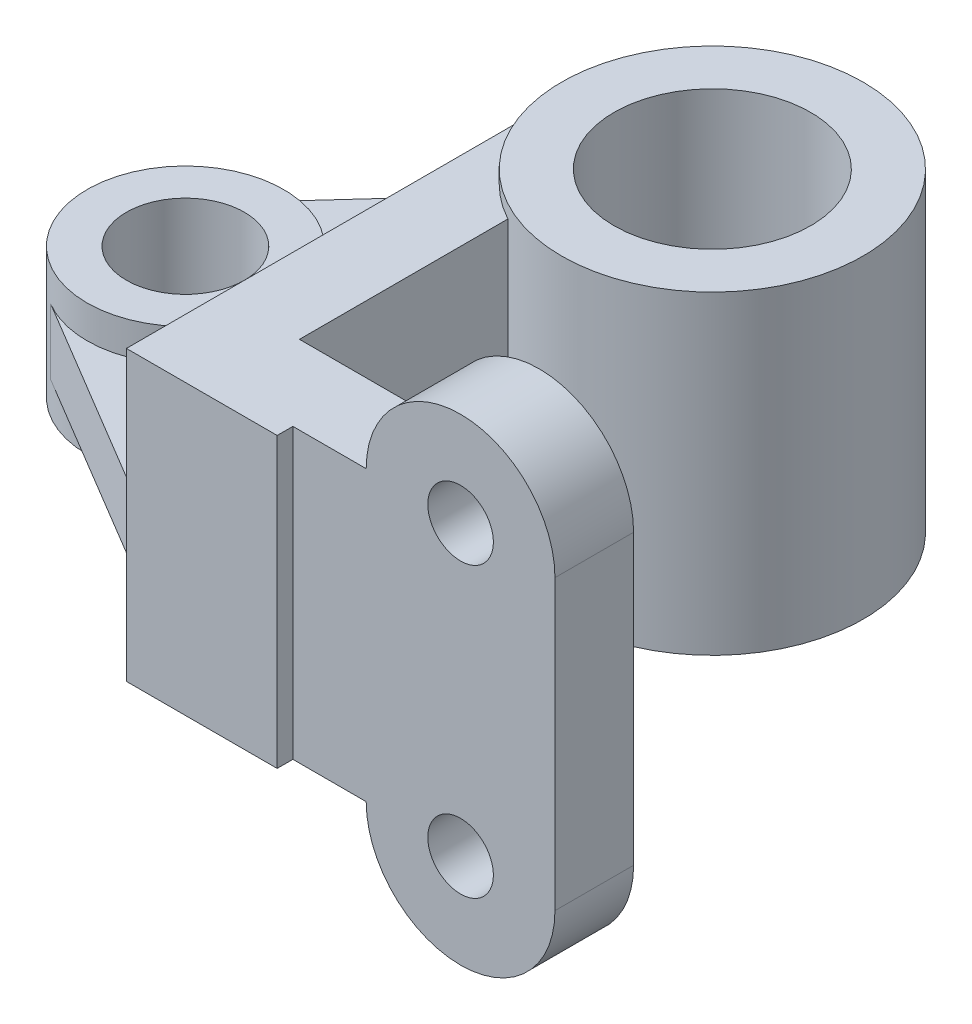
ISO-10303-21;
HEADER;
FILE_DESCRIPTION(('STEP AP214'),'2;1');
FILE_NAME('part.step','',(''),(''),'','','');
FILE_SCHEMA(('AUTOMOTIVE_DESIGN { 1 0 10303 214 1 1 1 1 }'));
ENDSEC;
DATA;
#1=APPLICATION_CONTEXT('core data for automotive mechanical design processes');
#2=APPLICATION_PROTOCOL_DEFINITION('international standard','automotive_design',2000,#1);
#3=PRODUCT_CONTEXT('',#1,'mechanical');
#4=PRODUCT('Part','Part','',(#3));
#5=PRODUCT_RELATED_PRODUCT_CATEGORY('part','',(#4));
#6=PRODUCT_DEFINITION_FORMATION('','',#4);
#7=PRODUCT_DEFINITION_CONTEXT('part definition',#1,'design');
#8=PRODUCT_DEFINITION('design','',#6,#7);
#9=PRODUCT_DEFINITION_SHAPE('','',#8);
#10=(LENGTH_UNIT() NAMED_UNIT(*) SI_UNIT(.MILLI.,.METRE.));
#11=(NAMED_UNIT(*) PLANE_ANGLE_UNIT() SI_UNIT($,.RADIAN.));
#12=(NAMED_UNIT(*) SI_UNIT($,.STERADIAN.) SOLID_ANGLE_UNIT());
#13=UNCERTAINTY_MEASURE_WITH_UNIT(LENGTH_MEASURE(1.E-05),#10,'distance_accuracy_value','');
#14=(GEOMETRIC_REPRESENTATION_CONTEXT(3) GLOBAL_UNCERTAINTY_ASSIGNED_CONTEXT((#13)) GLOBAL_UNIT_ASSIGNED_CONTEXT((#10,
#11,#12)) REPRESENTATION_CONTEXT('',''));
#15=CARTESIAN_POINT('',(0.,0.,0.));
#16=DIRECTION('',(0.,0.,1.));
#17=DIRECTION('',(1.,0.,0.));
#18=AXIS2_PLACEMENT_3D('',#15,#16,#17);
#19=CARTESIAN_POINT('',(55.2083333333334,-55.,0.));
#20=DIRECTION('',(0.,0.,1.));
#21=DIRECTION('',(1.,0.,0.));
#22=AXIS2_PLACEMENT_3D('',#19,#20,#21);
#23=PLANE('',#22);
#24=CARTESIAN_POINT('',(55.2083333333334,55.,0.));
#25=DIRECTION('',(0.,0.,1.));
#26=DIRECTION('',(1.,0.,0.));
#27=AXIS2_PLACEMENT_3D('',#24,#25,#26);
#28=CIRCLE('',#27,30.);
#29=CARTESIAN_POINT('',(85.2083333333334,55.,0.));
#30=VERTEX_POINT('',#29);
#31=EDGE_CURVE('E47',#30,#30,#28,.F.);
#32=ORIENTED_EDGE('',*,*,#31,.F.);
#33=EDGE_LOOP('',(#32));
#34=FACE_BOUND('',#33,.T.);
#35=DIRECTION('',(0.,-1.,0.));
#36=VECTOR('',#35,1.);
#37=CARTESIAN_POINT('',(-36.25,55.,0.));
#38=LINE('',#37,#36);
#39=CARTESIAN_POINT('',(-36.25,55.,0.));
#40=VERTEX_POINT('',#39);
#41=CARTESIAN_POINT('',(-36.25,-55.,0.));
#42=VERTEX_POINT('',#41);
#43=EDGE_CURVE('E212',#40,#42,#38,.T.);
#44=ORIENTED_EDGE('',*,*,#43,.F.);
#45=DIRECTION('',(-1.,0.,0.));
#46=VECTOR('',#45,1.);
#47=CARTESIAN_POINT('',(-66.25,55.,0.));
#48=LINE('',#47,#46);
#49=CARTESIAN_POINT('',(19.2083333333334,54.9999999999999,0.));
#50=VERTEX_POINT('',#49);
#51=EDGE_CURVE('E266',#50,#40,#48,.T.);
#52=ORIENTED_EDGE('',*,*,#51,.F.);
#53=CARTESIAN_POINT('',(55.2083333333334,55.,0.));
#54=DIRECTION('',(0.,0.,1.));
#55=DIRECTION('',(1.,0.,0.));
#56=AXIS2_PLACEMENT_3D('',#53,#54,#55);
#57=CIRCLE('',#56,36.);
#58=CARTESIAN_POINT('',(91.2083333333334,55.,0.));
#59=VERTEX_POINT('',#58);
#60=EDGE_CURVE('E263',#59,#50,#57,.T.);
#61=ORIENTED_EDGE('',*,*,#60,.F.);
#62=DIRECTION('',(0.,1.,0.));
#63=VECTOR('',#62,1.);
#64=CARTESIAN_POINT('',(91.2083333333334,55.,0.));
#65=LINE('',#64,#63);
#66=CARTESIAN_POINT('',(91.2083333333334,-55.0000000000001,0.));
#67=VERTEX_POINT('',#66);
#68=EDGE_CURVE('E257',#67,#59,#65,.T.);
#69=ORIENTED_EDGE('',*,*,#68,.F.);
#70=CARTESIAN_POINT('',(55.2083333333334,-55.,0.));
#71=DIRECTION('',(0.,0.,1.));
#72=DIRECTION('',(1.,0.,0.));
#73=AXIS2_PLACEMENT_3D('',#70,#71,#72);
#74=CIRCLE('',#73,36.);
#75=CARTESIAN_POINT('',(19.2083333333334,-55.,0.));
#76=VERTEX_POINT('',#75);
#77=EDGE_CURVE('E260',#76,#67,#74,.T.);
#78=ORIENTED_EDGE('',*,*,#77,.F.);
#79=DIRECTION('',(1.,0.,0.));
#80=VECTOR('',#79,1.);
#81=CARTESIAN_POINT('',(-66.2499999999999,-55.,0.));
#82=LINE('',#81,#80);
#83=EDGE_CURVE('E250',#42,#76,#82,.T.);
#84=ORIENTED_EDGE('',*,*,#83,.F.);
#85=EDGE_LOOP('',(#44,#52,#61,#69,#78,#84));
#86=FACE_BOUND('',#85,.T.);
#87=CARTESIAN_POINT('',(55.2083333333334,-55.,0.));
#88=DIRECTION('',(0.,0.,1.));
#89=DIRECTION('',(1.,0.,0.));
#90=AXIS2_PLACEMENT_3D('',#87,#88,#89);
#91=CIRCLE('',#90,30.);
#92=CARTESIAN_POINT('',(85.2083333333334,-55.,0.));
#93=VERTEX_POINT('',#92);
#94=EDGE_CURVE('E11',#93,#93,#91,.F.);
#95=ORIENTED_EDGE('',*,*,#94,.F.);
#96=EDGE_LOOP('',(#95));
#97=FACE_BOUND('',#96,.T.);
#98=ADVANCED_FACE('F41',(#34,#86,#97),#23,.F.);
#99=CARTESIAN_POINT('',(-66.25,55.,36.));
#100=DIRECTION('',(1.,0.,0.));
#101=DIRECTION('',(0.,1.,0.));
#102=AXIS2_PLACEMENT_3D('',#99,#100,#101);
#103=PLANE('',#102);
#104=DIRECTION('',(0.,0.,-1.));
#105=VECTOR('',#104,1.);
#106=CARTESIAN_POINT('',(-66.25,-12.5,36.));
#107=LINE('',#106,#105);
#108=CARTESIAN_POINT('',(-66.25,-12.5,36.));
#109=VERTEX_POINT('',#108);
#110=CARTESIAN_POINT('',(-66.25,-12.5,-130.));
#111=VERTEX_POINT('',#110);
#112=EDGE_CURVE('E159',#109,#111,#107,.T.);
#113=ORIENTED_EDGE('',*,*,#112,.T.);
#114=DIRECTION('',(0.,-1.,0.));
#115=VECTOR('',#114,1.);
#116=CARTESIAN_POINT('',(-66.25,55.,-130.));
#117=LINE('',#116,#115);
#118=CARTESIAN_POINT('',(-66.25,-55.,-130.));
#119=VERTEX_POINT('',#118);
#120=EDGE_CURVE('E220',#111,#119,#117,.T.);
#121=ORIENTED_EDGE('',*,*,#120,.T.);
#122=DIRECTION('',(0.,0.,-1.));
#123=VECTOR('',#122,1.);
#124=CARTESIAN_POINT('',(-66.2499999999999,-55.,36.));
#125=LINE('',#124,#123);
#126=CARTESIAN_POINT('',(-66.2499999999999,-55.,36.));
#127=VERTEX_POINT('',#126);
#128=EDGE_CURVE('E276',#127,#119,#125,.T.);
#129=ORIENTED_EDGE('',*,*,#128,.F.);
#130=DIRECTION('',(0.,-1.,0.));
#131=VECTOR('',#130,1.);
#132=CARTESIAN_POINT('',(-66.25,55.,36.));
#133=LINE('',#132,#131);
#134=EDGE_CURVE('E57',#109,#127,#133,.T.);
#135=ORIENTED_EDGE('',*,*,#134,.F.);
#136=EDGE_LOOP('',(#113,#121,#129,#135));
#137=FACE_BOUND('',#136,.T.);
#138=ADVANCED_FACE('F291',(#137),#103,.F.);
#139=CARTESIAN_POINT('',(55.2083333333334,-55.,36.));
#140=DIRECTION('',(0.,0.,1.));
#141=DIRECTION('',(1.,0.,0.));
#142=AXIS2_PLACEMENT_3D('',#139,#140,#141);
#143=PLANE('',#142);
#144=DIRECTION('',(0.,1.,0.));
#145=VECTOR('',#144,1.);
#146=CARTESIAN_POINT('',(-8.74999999999997,-118.,36.));
#147=LINE('',#146,#145);
#148=CARTESIAN_POINT('',(-8.74999999999997,-55.,36.));
#149=VERTEX_POINT('',#148);
#150=CARTESIAN_POINT('',(-8.74999999999997,54.9999999999999,36.));
#151=VERTEX_POINT('',#150);
#152=EDGE_CURVE('E222',#149,#151,#147,.T.);
#153=ORIENTED_EDGE('',*,*,#152,.T.);
#154=DIRECTION('',(-1.,0.,0.));
#155=VECTOR('',#154,1.);
#156=CARTESIAN_POINT('',(-66.25,55.,36.));
#157=LINE('',#156,#155);
#158=CARTESIAN_POINT('',(-66.25,55.,36.));
#159=VERTEX_POINT('',#158);
#160=EDGE_CURVE('E251',#151,#159,#157,.T.);
#161=ORIENTED_EDGE('',*,*,#160,.T.);
#162=CARTESIAN_POINT('',(-66.25,12.5,36.));
#163=VERTEX_POINT('',#162);
#164=EDGE_CURVE('E246',#159,#163,#133,.T.);
#165=ORIENTED_EDGE('',*,*,#164,.T.);
#166=DIRECTION('',(0.,-1.,0.));
#167=VECTOR('',#166,1.);
#168=CARTESIAN_POINT('',(-66.25,12.5,36.));
#169=LINE('',#168,#167);
#170=EDGE_CURVE('E173',#163,#109,#169,.T.);
#171=ORIENTED_EDGE('',*,*,#170,.T.);
#172=ORIENTED_EDGE('',*,*,#134,.T.);
#173=DIRECTION('',(1.,0.,0.));
#174=VECTOR('',#173,1.);
#175=CARTESIAN_POINT('',(-66.2499999999999,-55.,36.));
#176=LINE('',#175,#174);
#177=EDGE_CURVE('E247',#127,#149,#176,.T.);
#178=ORIENTED_EDGE('',*,*,#177,.T.);
#179=EDGE_LOOP('',(#153,#161,#165,#171,#172,#178));
#180=FACE_BOUND('',#179,.T.);
#181=ADVANCED_FACE('F381',(#180),#143,.T.);
#182=CARTESIAN_POINT('',(-66.25,55.,-130.));
#183=VERTEX_POINT('',#182);
#184=CARTESIAN_POINT('',(-66.25,12.5,-130.));
#185=VERTEX_POINT('',#184);
#186=EDGE_CURVE('E217',#183,#185,#117,.T.);
#187=ORIENTED_EDGE('',*,*,#186,.T.);
#188=DIRECTION('',(0.,0.,-1.));
#189=VECTOR('',#188,1.);
#190=CARTESIAN_POINT('',(-66.25,12.5,36.));
#191=LINE('',#190,#189);
#192=EDGE_CURVE('E64',#163,#185,#191,.T.);
#193=ORIENTED_EDGE('',*,*,#192,.F.);
#194=ORIENTED_EDGE('',*,*,#164,.F.);
#195=DIRECTION('',(0.,0.,-1.));
#196=VECTOR('',#195,1.);
#197=CARTESIAN_POINT('',(-66.25,55.,36.));
#198=LINE('',#197,#196);
#199=EDGE_CURVE('E254',#159,#183,#198,.T.);
#200=ORIENTED_EDGE('',*,*,#199,.T.);
#201=EDGE_LOOP('',(#187,#193,#194,#200));
#202=FACE_BOUND('',#201,.T.);
#203=ADVANCED_FACE('F43',(#202),#103,.F.);
#204=CARTESIAN_POINT('',(-66.2499999999999,-55.,36.));
#205=DIRECTION('',(0.,1.,0.));
#206=DIRECTION('',(0.,0.,1.));
#207=AXIS2_PLACEMENT_3D('',#204,#205,#206);
#208=PLANE('',#207);
#209=DIRECTION('',(-1.,0.,0.));
#210=VECTOR('',#209,1.);
#211=CARTESIAN_POINT('',(-66.2499999999999,-55.,30.));
#212=LINE('',#211,#210);
#213=CARTESIAN_POINT('',(19.2083333333334,-55.,30.));
#214=VERTEX_POINT('',#213);
#215=CARTESIAN_POINT('',(-8.74999999999997,-55.,30.));
#216=VERTEX_POINT('',#215);
#217=EDGE_CURVE('E242',#214,#216,#212,.T.);
#218=ORIENTED_EDGE('',*,*,#217,.T.);
#219=DIRECTION('',(0.,0.,1.));
#220=VECTOR('',#219,1.);
#221=CARTESIAN_POINT('',(-8.74999999999997,-55.,36.));
#222=LINE('',#221,#220);
#223=EDGE_CURVE('E244',#216,#149,#222,.T.);
#224=ORIENTED_EDGE('',*,*,#223,.T.);
#225=ORIENTED_EDGE('',*,*,#177,.F.);
#226=ORIENTED_EDGE('',*,*,#128,.T.);
#227=CARTESIAN_POINT('',(-8.74999999999997,-55.,-130.));
#228=DIRECTION('',(0.,1.,0.));
#229=DIRECTION('',(0.,0.,1.));
#230=AXIS2_PLACEMENT_3D('',#227,#228,#229);
#231=CIRCLE('',#230,57.5);
#232=CARTESIAN_POINT('',(-36.25,-55.,-79.5024753081896));
#233=VERTEX_POINT('',#232);
#234=EDGE_CURVE('E197',#119,#233,#231,.T.);
#235=ORIENTED_EDGE('',*,*,#234,.T.);
#236=DIRECTION('',(0.,0.,-1.));
#237=VECTOR('',#236,1.);
#238=CARTESIAN_POINT('',(-36.25,-55.,0.));
#239=LINE('',#238,#237);
#240=EDGE_CURVE('E206',#42,#233,#239,.T.);
#241=ORIENTED_EDGE('',*,*,#240,.F.);
#242=ORIENTED_EDGE('',*,*,#83,.T.);
#243=DIRECTION('',(0.,0.,-1.));
#244=VECTOR('',#243,1.);
#245=CARTESIAN_POINT('',(19.2083333333334,-55.,36.));
#246=LINE('',#245,#244);
#247=EDGE_CURVE('E277',#214,#76,#246,.T.);
#248=ORIENTED_EDGE('',*,*,#247,.F.);
#249=EDGE_LOOP('',(#218,#224,#225,#226,#235,#241,#242,#248));
#250=FACE_BOUND('',#249,.T.);
#251=ADVANCED_FACE('F396',(#250),#208,.F.);
#252=CARTESIAN_POINT('',(55.2083333333334,-55.,36.));
#253=DIRECTION('',(0.,0.,-1.));
#254=DIRECTION('',(-1.,0.,0.));
#255=AXIS2_PLACEMENT_3D('',#252,#253,#254);
#256=CYLINDRICAL_SURFACE('',#255,36.);
#257=DIRECTION('',(0.,0.,-1.));
#258=VECTOR('',#257,1.);
#259=CARTESIAN_POINT('',(91.2083333333334,-55.0000000000001,36.));
#260=LINE('',#259,#258);
#261=CARTESIAN_POINT('',(91.2083333333334,-55.0000000000001,30.));
#262=VERTEX_POINT('',#261);
#263=EDGE_CURVE('E273',#262,#67,#260,.T.);
#264=ORIENTED_EDGE('',*,*,#263,.F.);
#265=CARTESIAN_POINT('',(55.2083333333334,-55.,30.));
#266=DIRECTION('',(0.,0.,-1.));
#267=DIRECTION('',(-1.,0.,0.));
#268=AXIS2_PLACEMENT_3D('',#265,#266,#267);
#269=CIRCLE('',#268,36.);
#270=EDGE_CURVE('E236',#262,#214,#269,.T.);
#271=ORIENTED_EDGE('',*,*,#270,.T.);
#272=ORIENTED_EDGE('',*,*,#247,.T.);
#273=ORIENTED_EDGE('',*,*,#77,.T.);
#274=EDGE_LOOP('',(#264,#271,#272,#273));
#275=FACE_BOUND('',#274,.T.);
#276=ADVANCED_FACE('F391',(#275),#256,.T.);
#277=CARTESIAN_POINT('',(91.2083333333334,55.,36.));
#278=DIRECTION('',(-1.,0.,0.));
#279=DIRECTION('',(0.,-1.,0.));
#280=AXIS2_PLACEMENT_3D('',#277,#278,#279);
#281=PLANE('',#280);
#282=DIRECTION('',(0.,0.,-1.));
#283=VECTOR('',#282,1.);
#284=CARTESIAN_POINT('',(91.2083333333334,55.,36.));
#285=LINE('',#284,#283);
#286=CARTESIAN_POINT('',(91.2083333333334,55.,30.));
#287=VERTEX_POINT('',#286);
#288=EDGE_CURVE('E275',#287,#59,#285,.T.);
#289=ORIENTED_EDGE('',*,*,#288,.F.);
#290=DIRECTION('',(0.,1.,0.));
#291=VECTOR('',#290,1.);
#292=CARTESIAN_POINT('',(91.2083333333334,-118.,30.));
#293=LINE('',#292,#291);
#294=EDGE_CURVE('E219',#262,#287,#293,.T.);
#295=ORIENTED_EDGE('',*,*,#294,.F.);
#296=ORIENTED_EDGE('',*,*,#263,.T.);
#297=ORIENTED_EDGE('',*,*,#68,.T.);
#298=EDGE_LOOP('',(#289,#295,#296,#297));
#299=FACE_BOUND('',#298,.T.);
#300=ADVANCED_FACE('F392',(#299),#281,.F.);
#301=CARTESIAN_POINT('',(55.2083333333334,55.,36.));
#302=DIRECTION('',(0.,0.,-1.));
#303=DIRECTION('',(-1.,0.,0.));
#304=AXIS2_PLACEMENT_3D('',#301,#302,#303);
#305=CYLINDRICAL_SURFACE('',#304,36.);
#306=DIRECTION('',(0.,0.,-1.));
#307=VECTOR('',#306,1.);
#308=CARTESIAN_POINT('',(19.2083333333334,54.9999999999999,36.));
#309=LINE('',#308,#307);
#310=CARTESIAN_POINT('',(19.2083333333334,54.9999999999999,30.));
#311=VERTEX_POINT('',#310);
#312=EDGE_CURVE('E269',#311,#50,#309,.T.);
#313=ORIENTED_EDGE('',*,*,#312,.F.);
#314=CARTESIAN_POINT('',(55.2083333333334,55.,30.));
#315=DIRECTION('',(0.,0.,-1.));
#316=DIRECTION('',(-1.,0.,0.));
#317=AXIS2_PLACEMENT_3D('',#314,#315,#316);
#318=CIRCLE('',#317,36.);
#319=EDGE_CURVE('E232',#311,#287,#318,.T.);
#320=ORIENTED_EDGE('',*,*,#319,.T.);
#321=ORIENTED_EDGE('',*,*,#288,.T.);
#322=ORIENTED_EDGE('',*,*,#60,.T.);
#323=EDGE_LOOP('',(#313,#320,#321,#322));
#324=FACE_BOUND('',#323,.T.);
#325=ADVANCED_FACE('F390',(#324),#305,.T.);
#326=CARTESIAN_POINT('',(-66.25,55.,36.));
#327=DIRECTION('',(0.,-1.,0.));
#328=DIRECTION('',(1.,0.,0.));
#329=AXIS2_PLACEMENT_3D('',#326,#327,#328);
#330=PLANE('',#329);
#331=ORIENTED_EDGE('',*,*,#160,.F.);
#332=DIRECTION('',(0.,0.,-1.));
#333=VECTOR('',#332,1.);
#334=CARTESIAN_POINT('',(-8.74999999999997,54.9999999999999,36.));
#335=LINE('',#334,#333);
#336=CARTESIAN_POINT('',(-8.74999999999997,54.9999999999999,30.));
#337=VERTEX_POINT('',#336);
#338=EDGE_CURVE('E285',#151,#337,#335,.T.);
#339=ORIENTED_EDGE('',*,*,#338,.T.);
#340=DIRECTION('',(1.,0.,0.));
#341=VECTOR('',#340,1.);
#342=CARTESIAN_POINT('',(-66.25,55.,30.));
#343=LINE('',#342,#341);
#344=EDGE_CURVE('E235',#337,#311,#343,.T.);
#345=ORIENTED_EDGE('',*,*,#344,.T.);
#346=ORIENTED_EDGE('',*,*,#312,.T.);
#347=ORIENTED_EDGE('',*,*,#51,.T.);
#348=DIRECTION('',(0.,0.,-1.));
#349=VECTOR('',#348,1.);
#350=CARTESIAN_POINT('',(-36.25,55.,0.));
#351=LINE('',#350,#349);
#352=CARTESIAN_POINT('',(-36.25,55.,-79.5024753081896));
#353=VERTEX_POINT('',#352);
#354=EDGE_CURVE('E202',#40,#353,#351,.T.);
#355=ORIENTED_EDGE('',*,*,#354,.T.);
#356=CARTESIAN_POINT('',(-8.74999999999997,55.,-130.));
#357=DIRECTION('',(0.,1.,0.));
#358=DIRECTION('',(0.,0.,1.));
#359=AXIS2_PLACEMENT_3D('',#356,#357,#358);
#360=CIRCLE('',#359,57.5);
#361=EDGE_CURVE('E205',#183,#353,#360,.T.);
#362=ORIENTED_EDGE('',*,*,#361,.F.);
#363=ORIENTED_EDGE('',*,*,#199,.F.);
#364=EDGE_LOOP('',(#331,#339,#345,#346,#347,#355,#362,#363));
#365=FACE_BOUND('',#364,.T.);
#366=ADVANCED_FACE('F377',(#365),#330,.F.);
#367=CARTESIAN_POINT('',(55.2083333333334,55.,36.));
#368=DIRECTION('',(0.,0.,-1.));
#369=DIRECTION('',(-1.,0.,0.));
#370=AXIS2_PLACEMENT_3D('',#367,#368,#369);
#371=CYLINDRICAL_SURFACE('',#370,12.5);
#372=CARTESIAN_POINT('',(55.2083333333334,55.,30.));
#373=DIRECTION('',(0.,0.,-1.));
#374=DIRECTION('',(-1.,0.,0.));
#375=AXIS2_PLACEMENT_3D('',#372,#373,#374);
#376=CIRCLE('',#375,12.5);
#377=CARTESIAN_POINT('',(42.7083333333334,55.,30.));
#378=VERTEX_POINT('',#377);
#379=EDGE_CURVE('E229',#378,#378,#376,.T.);
#380=ORIENTED_EDGE('',*,*,#379,.F.);
#381=EDGE_LOOP('',(#380));
#382=FACE_BOUND('',#381,.T.);
#383=CARTESIAN_POINT('',(55.2083333333334,55.,-3.));
#384=DIRECTION('',(0.,0.,-1.));
#385=DIRECTION('',(-1.,0.,0.));
#386=AXIS2_PLACEMENT_3D('',#383,#384,#385);
#387=CIRCLE('',#386,12.5);
#388=CARTESIAN_POINT('',(42.7083333333334,55.,-3.));
#389=VERTEX_POINT('',#388);
#390=EDGE_CURVE('E446',#389,#389,#387,.T.);
#391=ORIENTED_EDGE('',*,*,#390,.T.);
#392=EDGE_LOOP('',(#391));
#393=FACE_BOUND('',#392,.T.);
#394=ADVANCED_FACE('F374',(#382,#393),#371,.F.);
#395=CARTESIAN_POINT('',(55.2083333333334,-55.,36.));
#396=DIRECTION('',(0.,0.,-1.));
#397=DIRECTION('',(-1.,0.,0.));
#398=AXIS2_PLACEMENT_3D('',#395,#396,#397);
#399=CYLINDRICAL_SURFACE('',#398,12.5);
#400=CARTESIAN_POINT('',(55.2083333333334,-55.,30.));
#401=DIRECTION('',(0.,0.,-1.));
#402=DIRECTION('',(-1.,0.,0.));
#403=AXIS2_PLACEMENT_3D('',#400,#401,#402);
#404=CIRCLE('',#403,12.5);
#405=CARTESIAN_POINT('',(42.7083333333334,-55.,30.));
#406=VERTEX_POINT('',#405);
#407=EDGE_CURVE('E221',#406,#406,#404,.T.);
#408=ORIENTED_EDGE('',*,*,#407,.F.);
#409=EDGE_LOOP('',(#408));
#410=FACE_BOUND('',#409,.T.);
#411=CARTESIAN_POINT('',(55.2083333333334,-55.,-3.));
#412=DIRECTION('',(0.,0.,-1.));
#413=DIRECTION('',(-1.,0.,0.));
#414=AXIS2_PLACEMENT_3D('',#411,#412,#413);
#415=CIRCLE('',#414,12.5);
#416=CARTESIAN_POINT('',(42.7083333333334,-55.,-3.));
#417=VERTEX_POINT('',#416);
#418=EDGE_CURVE('E457',#417,#417,#415,.T.);
#419=ORIENTED_EDGE('',*,*,#418,.T.);
#420=EDGE_LOOP('',(#419));
#421=FACE_BOUND('',#420,.T.);
#422=ADVANCED_FACE('F366',(#410,#421),#399,.F.);
#423=CARTESIAN_POINT('',(-8.74999999999997,-118.,36.));
#424=DIRECTION('',(-1.,0.,0.));
#425=DIRECTION('',(0.,0.,1.));
#426=AXIS2_PLACEMENT_3D('',#423,#424,#425);
#427=PLANE('',#426);
#428=DIRECTION('',(0.,1.,0.));
#429=VECTOR('',#428,1.);
#430=CARTESIAN_POINT('',(-8.74999999999997,-118.,30.));
#431=LINE('',#430,#429);
#432=EDGE_CURVE('E223',#216,#337,#431,.T.);
#433=ORIENTED_EDGE('',*,*,#432,.T.);
#434=ORIENTED_EDGE('',*,*,#338,.F.);
#435=ORIENTED_EDGE('',*,*,#152,.F.);
#436=ORIENTED_EDGE('',*,*,#223,.F.);
#437=EDGE_LOOP('',(#433,#434,#435,#436));
#438=FACE_BOUND('',#437,.T.);
#439=ADVANCED_FACE('F364',(#438),#427,.F.);
#440=CARTESIAN_POINT('',(-8.74999999999997,-118.,30.));
#441=DIRECTION('',(0.,0.,-1.));
#442=DIRECTION('',(-1.,0.,0.));
#443=AXIS2_PLACEMENT_3D('',#440,#441,#442);
#444=PLANE('',#443);
#445=ORIENTED_EDGE('',*,*,#379,.T.);
#446=EDGE_LOOP('',(#445));
#447=FACE_BOUND('',#446,.T.);
#448=ORIENTED_EDGE('',*,*,#407,.T.);
#449=EDGE_LOOP('',(#448));
#450=FACE_BOUND('',#449,.T.);
#451=ORIENTED_EDGE('',*,*,#270,.F.);
#452=ORIENTED_EDGE('',*,*,#294,.T.);
#453=ORIENTED_EDGE('',*,*,#319,.F.);
#454=ORIENTED_EDGE('',*,*,#344,.F.);
#455=ORIENTED_EDGE('',*,*,#432,.F.);
#456=ORIENTED_EDGE('',*,*,#217,.F.);
#457=EDGE_LOOP('',(#451,#452,#453,#454,#455,#456));
#458=FACE_BOUND('',#457,.T.);
#459=ADVANCED_FACE('F361',(#447,#450,#458),#444,.F.);
#460=CARTESIAN_POINT('',(-36.25,55.,0.));
#461=DIRECTION('',(-1.,0.,0.));
#462=DIRECTION('',(0.,0.,1.));
#463=AXIS2_PLACEMENT_3D('',#460,#461,#462);
#464=PLANE('',#463);
#465=ORIENTED_EDGE('',*,*,#240,.T.);
#466=DIRECTION('',(0.,-1.,0.));
#467=VECTOR('',#466,1.);
#468=CARTESIAN_POINT('',(-36.25,55.,-79.5024753081896));
#469=LINE('',#468,#467);
#470=EDGE_CURVE('E208',#353,#233,#469,.T.);
#471=ORIENTED_EDGE('',*,*,#470,.F.);
#472=ORIENTED_EDGE('',*,*,#354,.F.);
#473=ORIENTED_EDGE('',*,*,#43,.T.);
#474=EDGE_LOOP('',(#465,#471,#472,#473));
#475=FACE_BOUND('',#474,.T.);
#476=ADVANCED_FACE('F358',(#475),#464,.F.);
#477=CARTESIAN_POINT('',(-8.74999999999997,60.,-130.));
#478=DIRECTION('',(0.,-1.,0.));
#479=DIRECTION('',(0.,0.,-1.));
#480=AXIS2_PLACEMENT_3D('',#477,#478,#479);
#481=CYLINDRICAL_SURFACE('',#480,57.5);
#482=CARTESIAN_POINT('',(-8.74999999999997,60.,-130.));
#483=DIRECTION('',(0.,1.,0.));
#484=DIRECTION('',(0.,0.,1.));
#485=AXIS2_PLACEMENT_3D('',#482,#483,#484);
#486=CIRCLE('',#485,57.5);
#487=CARTESIAN_POINT('',(-8.74999999999997,60.,-72.5));
#488=VERTEX_POINT('',#487);
#489=EDGE_CURVE('E191',#488,#488,#486,.T.);
#490=ORIENTED_EDGE('',*,*,#489,.F.);
#491=EDGE_LOOP('',(#490));
#492=FACE_BOUND('',#491,.T.);
#493=CARTESIAN_POINT('',(-8.74999999999997,-60.,-130.));
#494=DIRECTION('',(0.,1.,0.));
#495=DIRECTION('',(0.,0.,1.));
#496=AXIS2_PLACEMENT_3D('',#493,#494,#495);
#497=CIRCLE('',#496,57.5);
#498=CARTESIAN_POINT('',(-8.74999999999997,-60.,-72.5));
#499=VERTEX_POINT('',#498);
#500=EDGE_CURVE('E194',#499,#499,#497,.T.);
#501=ORIENTED_EDGE('',*,*,#500,.T.);
#502=EDGE_LOOP('',(#501));
#503=FACE_BOUND('',#502,.T.);
#504=DIRECTION('',(0.,-1.,0.));
#505=VECTOR('',#504,1.);
#506=CARTESIAN_POINT('',(-51.2472115720593,12.5,-168.732893109083));
#507=LINE('',#506,#505);
#508=CARTESIAN_POINT('',(-51.2472115720593,12.5,-168.732893109083));
#509=VERTEX_POINT('',#508);
#510=CARTESIAN_POINT('',(-51.2472115720593,-12.5,-168.732893109083));
#511=VERTEX_POINT('',#510);
#512=EDGE_CURVE('E187',#509,#511,#507,.T.);
#513=ORIENTED_EDGE('',*,*,#512,.F.);
#514=CARTESIAN_POINT('',(-8.74999999999997,12.5,-130.));
#515=DIRECTION('',(0.,-1.,0.));
#516=DIRECTION('',(0.,0.,1.));
#517=AXIS2_PLACEMENT_3D('',#514,#515,#516);
#518=CIRCLE('',#517,57.5);
#519=EDGE_CURVE('E435',#185,#509,#518,.T.);
#520=ORIENTED_EDGE('',*,*,#519,.F.);
#521=ORIENTED_EDGE('',*,*,#186,.F.);
#522=ORIENTED_EDGE('',*,*,#361,.T.);
#523=ORIENTED_EDGE('',*,*,#470,.T.);
#524=ORIENTED_EDGE('',*,*,#234,.F.);
#525=ORIENTED_EDGE('',*,*,#120,.F.);
#526=CARTESIAN_POINT('',(-8.74999999999997,-12.5,-130.));
#527=DIRECTION('',(0.,-1.,0.));
#528=DIRECTION('',(0.,0.,1.));
#529=AXIS2_PLACEMENT_3D('',#526,#527,#528);
#530=CIRCLE('',#529,57.5);
#531=EDGE_CURVE('E177',#111,#511,#530,.T.);
#532=ORIENTED_EDGE('',*,*,#531,.T.);
#533=EDGE_LOOP('',(#513,#520,#521,#522,#523,#524,#525,#532));
#534=FACE_BOUND('',#533,.T.);
#535=ADVANCED_FACE('F353',(#492,#503,#534),#481,.T.);
#536=CARTESIAN_POINT('',(-8.74999999999997,60.,-130.));
#537=DIRECTION('',(0.,-1.,0.));
#538=DIRECTION('',(0.,0.,-1.));
#539=AXIS2_PLACEMENT_3D('',#536,#537,#538);
#540=CYLINDRICAL_SURFACE('',#539,37.5);
#541=CARTESIAN_POINT('',(-8.74999999999997,60.,-130.));
#542=DIRECTION('',(0.,1.,0.));
#543=DIRECTION('',(0.,0.,1.));
#544=AXIS2_PLACEMENT_3D('',#541,#542,#543);
#545=CIRCLE('',#544,37.5);
#546=CARTESIAN_POINT('',(-8.74999999999997,60.,-92.5));
#547=VERTEX_POINT('',#546);
#548=EDGE_CURVE('E186',#547,#547,#545,.T.);
#549=ORIENTED_EDGE('',*,*,#548,.T.);
#550=EDGE_LOOP('',(#549));
#551=FACE_BOUND('',#550,.T.);
#552=CARTESIAN_POINT('',(-8.74999999999997,-60.,-130.));
#553=DIRECTION('',(0.,1.,0.));
#554=DIRECTION('',(0.,0.,1.));
#555=AXIS2_PLACEMENT_3D('',#552,#553,#554);
#556=CIRCLE('',#555,37.5);
#557=CARTESIAN_POINT('',(-8.74999999999997,-60.,-92.5));
#558=VERTEX_POINT('',#557);
#559=EDGE_CURVE('E189',#558,#558,#556,.T.);
#560=ORIENTED_EDGE('',*,*,#559,.F.);
#561=EDGE_LOOP('',(#560));
#562=FACE_BOUND('',#561,.T.);
#563=ADVANCED_FACE('F346',(#551,#562),#540,.F.);
#564=CARTESIAN_POINT('',(0.,60.,0.));
#565=DIRECTION('',(0.,1.,0.));
#566=DIRECTION('',(0.,0.,1.));
#567=AXIS2_PLACEMENT_3D('',#564,#565,#566);
#568=PLANE('',#567);
#569=ORIENTED_EDGE('',*,*,#548,.F.);
#570=EDGE_LOOP('',(#569));
#571=FACE_BOUND('',#570,.T.);
#572=ORIENTED_EDGE('',*,*,#489,.T.);
#573=EDGE_LOOP('',(#572));
#574=FACE_BOUND('',#573,.T.);
#575=ADVANCED_FACE('F342',(#571,#574),#568,.T.);
#576=CARTESIAN_POINT('',(0.,-60.,0.));
#577=DIRECTION('',(0.,1.,0.));
#578=DIRECTION('',(0.,0.,1.));
#579=AXIS2_PLACEMENT_3D('',#576,#577,#578);
#580=PLANE('',#579);
#581=ORIENTED_EDGE('',*,*,#559,.T.);
#582=EDGE_LOOP('',(#581));
#583=FACE_BOUND('',#582,.T.);
#584=ORIENTED_EDGE('',*,*,#500,.F.);
#585=EDGE_LOOP('',(#584));
#586=FACE_BOUND('',#585,.T.);
#587=ADVANCED_FACE('F341',(#583,#586),#580,.F.);
#588=CARTESIAN_POINT('',(-146.465572764387,12.5,-64.2605824624453));
#589=DIRECTION('',(0.73908194038364,0.,0.673615532331873));
#590=DIRECTION('',(0.673615532331873,0.,-0.73908194038364));
#591=AXIS2_PLACEMENT_3D('',#588,#589,#590);
#592=PLANE('',#591);
#593=DIRECTION('',(-0.673615532331873,0.,0.73908194038364));
#594=VECTOR('',#593,1.);
#595=CARTESIAN_POINT('',(-146.465572764387,-12.5,-64.2605824624453));
#596=LINE('',#595,#594);
#597=CARTESIAN_POINT('',(-146.465572764386,-12.5,-64.2605824624453));
#598=VERTEX_POINT('',#597);
#599=EDGE_CURVE('E176',#511,#598,#596,.T.);
#600=ORIENTED_EDGE('',*,*,#599,.T.);
#601=DIRECTION('',(0.,-1.,0.));
#602=VECTOR('',#601,1.);
#603=CARTESIAN_POINT('',(-146.465572764386,12.5,-64.2605824624453));
#604=LINE('',#603,#602);
#605=CARTESIAN_POINT('',(-146.465572764386,12.5,-64.2605824624453));
#606=VERTEX_POINT('',#605);
#607=EDGE_CURVE('E175',#606,#598,#604,.T.);
#608=ORIENTED_EDGE('',*,*,#607,.F.);
#609=DIRECTION('',(-0.673615532331873,0.,0.73908194038364));
#610=VECTOR('',#609,1.);
#611=CARTESIAN_POINT('',(-146.465572764387,12.5,-64.2605824624453));
#612=LINE('',#611,#610);
#613=EDGE_CURVE('E424',#509,#606,#612,.T.);
#614=ORIENTED_EDGE('',*,*,#613,.F.);
#615=ORIENTED_EDGE('',*,*,#512,.T.);
#616=EDGE_LOOP('',(#600,#608,#614,#615));
#617=FACE_BOUND('',#616,.T.);
#618=ADVANCED_FACE('F336',(#617),#592,.F.);
#619=CARTESIAN_POINT('',(-137.966934712232,12.5,-6.79814570143782));
#620=DIRECTION('',(0.512451592326177,0.,-0.858716114628324));
#621=DIRECTION('',(-0.858716114628324,0.,-0.512451592326177));
#622=AXIS2_PLACEMENT_3D('',#619,#620,#621);
#623=PLANE('',#622);
#624=DIRECTION('',(0.858716114628324,0.,0.512451592326177));
#625=VECTOR('',#624,1.);
#626=CARTESIAN_POINT('',(-137.966934712232,-12.5,-6.79814570143782));
#627=LINE('',#626,#625);
#628=CARTESIAN_POINT('',(-137.966934712232,-12.5,-6.79814570143782));
#629=VERTEX_POINT('',#628);
#630=EDGE_CURVE('E155',#629,#109,#627,.T.);
#631=ORIENTED_EDGE('',*,*,#630,.T.);
#632=ORIENTED_EDGE('',*,*,#170,.F.);
#633=DIRECTION('',(0.858716114628324,0.,0.512451592326177));
#634=VECTOR('',#633,1.);
#635=CARTESIAN_POINT('',(-137.966934712232,12.5,-6.79814570143782));
#636=LINE('',#635,#634);
#637=CARTESIAN_POINT('',(-137.966934712232,12.5,-6.79814570143782));
#638=VERTEX_POINT('',#637);
#639=EDGE_CURVE('E166',#638,#163,#636,.T.);
#640=ORIENTED_EDGE('',*,*,#639,.F.);
#641=DIRECTION('',(0.,-1.,0.));
#642=VECTOR('',#641,1.);
#643=CARTESIAN_POINT('',(-137.966934712232,12.5,-6.79814570143782));
#644=LINE('',#643,#642);
#645=EDGE_CURVE('E167',#638,#629,#644,.T.);
#646=ORIENTED_EDGE('',*,*,#645,.T.);
#647=EDGE_LOOP('',(#631,#632,#640,#646));
#648=FACE_BOUND('',#647,.T.);
#649=ADVANCED_FACE('F170',(#648),#623,.F.);
#650=CARTESIAN_POINT('',(-8.74999999999997,12.5,-130.));
#651=DIRECTION('',(0.,1.,0.));
#652=DIRECTION('',(0.,0.,1.));
#653=AXIS2_PLACEMENT_3D('',#650,#651,#652);
#654=PLANE('',#653);
#655=ORIENTED_EDGE('',*,*,#192,.T.);
#656=ORIENTED_EDGE('',*,*,#519,.T.);
#657=ORIENTED_EDGE('',*,*,#613,.T.);
#658=CARTESIAN_POINT('',(-118.75,12.5,-39.));
#659=DIRECTION('',(0.,-1.,0.));
#660=DIRECTION('',(0.,0.,1.));
#661=AXIS2_PLACEMENT_3D('',#658,#659,#660);
#662=CIRCLE('',#661,37.5);
#663=EDGE_CURVE('E425',#606,#638,#662,.T.);
#664=ORIENTED_EDGE('',*,*,#663,.T.);
#665=ORIENTED_EDGE('',*,*,#639,.T.);
#666=EDGE_LOOP('',(#655,#656,#657,#664,#665));
#667=FACE_BOUND('',#666,.T.);
#668=ADVANCED_FACE('F335',(#667),#654,.T.);
#669=CARTESIAN_POINT('',(-8.74999999999997,-12.5,-130.));
#670=DIRECTION('',(0.,1.,0.));
#671=DIRECTION('',(0.,0.,1.));
#672=AXIS2_PLACEMENT_3D('',#669,#670,#671);
#673=PLANE('',#672);
#674=ORIENTED_EDGE('',*,*,#112,.F.);
#675=ORIENTED_EDGE('',*,*,#630,.F.);
#676=CARTESIAN_POINT('',(-118.75,-12.5,-39.));
#677=DIRECTION('',(0.,-1.,0.));
#678=DIRECTION('',(0.,0.,1.));
#679=AXIS2_PLACEMENT_3D('',#676,#677,#678);
#680=CIRCLE('',#679,37.5);
#681=EDGE_CURVE('E160',#598,#629,#680,.T.);
#682=ORIENTED_EDGE('',*,*,#681,.F.);
#683=ORIENTED_EDGE('',*,*,#599,.F.);
#684=ORIENTED_EDGE('',*,*,#531,.F.);
#685=EDGE_LOOP('',(#674,#675,#682,#683,#684));
#686=FACE_BOUND('',#685,.T.);
#687=ADVANCED_FACE('F152',(#686),#673,.F.);
#688=CARTESIAN_POINT('',(-118.75,25.,-39.));
#689=DIRECTION('',(0.,-1.,0.));
#690=DIRECTION('',(0.,0.,-1.));
#691=AXIS2_PLACEMENT_3D('',#688,#689,#690);
#692=CYLINDRICAL_SURFACE('',#691,22.5);
#693=CARTESIAN_POINT('',(-118.75,25.,-39.));
#694=DIRECTION('',(0.,1.,0.));
#695=DIRECTION('',(0.,0.,1.));
#696=AXIS2_PLACEMENT_3D('',#693,#694,#695);
#697=CIRCLE('',#696,22.5);
#698=CARTESIAN_POINT('',(-118.75,25.,-16.5));
#699=VERTEX_POINT('',#698);
#700=EDGE_CURVE('E438',#699,#699,#697,.T.);
#701=ORIENTED_EDGE('',*,*,#700,.T.);
#702=EDGE_LOOP('',(#701));
#703=FACE_BOUND('',#702,.T.);
#704=CARTESIAN_POINT('',(-118.75,-25.,-39.));
#705=DIRECTION('',(0.,1.,0.));
#706=DIRECTION('',(0.,0.,1.));
#707=AXIS2_PLACEMENT_3D('',#704,#705,#706);
#708=CIRCLE('',#707,22.5);
#709=CARTESIAN_POINT('',(-118.75,-25.,-16.5));
#710=VERTEX_POINT('',#709);
#711=EDGE_CURVE('E439',#710,#710,#708,.T.);
#712=ORIENTED_EDGE('',*,*,#711,.F.);
#713=EDGE_LOOP('',(#712));
#714=FACE_BOUND('',#713,.T.);
#715=ADVANCED_FACE('F327',(#703,#714),#692,.F.);
#716=CARTESIAN_POINT('',(-118.75,25.,-39.));
#717=DIRECTION('',(0.,-1.,0.));
#718=DIRECTION('',(0.,0.,-1.));
#719=AXIS2_PLACEMENT_3D('',#716,#717,#718);
#720=CYLINDRICAL_SURFACE('',#719,37.5);
#721=ORIENTED_EDGE('',*,*,#663,.F.);
#722=ORIENTED_EDGE('',*,*,#607,.T.);
#723=ORIENTED_EDGE('',*,*,#681,.T.);
#724=ORIENTED_EDGE('',*,*,#645,.F.);
#725=EDGE_LOOP('',(#721,#722,#723,#724));
#726=FACE_BOUND('',#725,.T.);
#727=CARTESIAN_POINT('',(-118.75,25.,-39.));
#728=DIRECTION('',(0.,1.,0.));
#729=DIRECTION('',(0.,0.,1.));
#730=AXIS2_PLACEMENT_3D('',#727,#728,#729);
#731=CIRCLE('',#730,37.5);
#732=CARTESIAN_POINT('',(-118.75,25.,-1.49999999999999));
#733=VERTEX_POINT('',#732);
#734=EDGE_CURVE('E428',#733,#733,#731,.T.);
#735=ORIENTED_EDGE('',*,*,#734,.F.);
#736=EDGE_LOOP('',(#735));
#737=FACE_BOUND('',#736,.T.);
#738=CARTESIAN_POINT('',(-118.75,-25.,-39.));
#739=DIRECTION('',(0.,1.,0.));
#740=DIRECTION('',(0.,0.,1.));
#741=AXIS2_PLACEMENT_3D('',#738,#739,#740);
#742=CIRCLE('',#741,37.5);
#743=CARTESIAN_POINT('',(-118.75,-25.,-1.49999999999999));
#744=VERTEX_POINT('',#743);
#745=EDGE_CURVE('E436',#744,#744,#742,.T.);
#746=ORIENTED_EDGE('',*,*,#745,.T.);
#747=EDGE_LOOP('',(#746));
#748=FACE_BOUND('',#747,.T.);
#749=ADVANCED_FACE('F171',(#726,#737,#748),#720,.T.);
#750=CARTESIAN_POINT('',(0.,25.,0.));
#751=DIRECTION('',(0.,1.,0.));
#752=DIRECTION('',(0.,0.,1.));
#753=AXIS2_PLACEMENT_3D('',#750,#751,#752);
#754=PLANE('',#753);
#755=ORIENTED_EDGE('',*,*,#700,.F.);
#756=EDGE_LOOP('',(#755));
#757=FACE_BOUND('',#756,.T.);
#758=ORIENTED_EDGE('',*,*,#734,.T.);
#759=EDGE_LOOP('',(#758));
#760=FACE_BOUND('',#759,.T.);
#761=ADVANCED_FACE('F317',(#757,#760),#754,.T.);
#762=CARTESIAN_POINT('',(0.,-25.,0.));
#763=DIRECTION('',(0.,1.,0.));
#764=DIRECTION('',(0.,0.,1.));
#765=AXIS2_PLACEMENT_3D('',#762,#763,#764);
#766=PLANE('',#765);
#767=ORIENTED_EDGE('',*,*,#711,.T.);
#768=EDGE_LOOP('',(#767));
#769=FACE_BOUND('',#768,.T.);
#770=ORIENTED_EDGE('',*,*,#745,.F.);
#771=EDGE_LOOP('',(#770));
#772=FACE_BOUND('',#771,.T.);
#773=ADVANCED_FACE('F320',(#769,#772),#766,.F.);
#774=CARTESIAN_POINT('',(55.2083333333334,55.,-3.));
#775=DIRECTION('',(0.,0.,1.));
#776=DIRECTION('',(1.,0.,0.));
#777=AXIS2_PLACEMENT_3D('',#774,#775,#776);
#778=CYLINDRICAL_SURFACE('',#777,30.);
#779=CARTESIAN_POINT('',(55.2083333333334,55.,-3.));
#780=DIRECTION('',(0.,0.,-1.));
#781=DIRECTION('',(-1.,0.,0.));
#782=AXIS2_PLACEMENT_3D('',#779,#780,#781);
#783=CIRCLE('',#782,30.);
#784=CARTESIAN_POINT('',(25.2083333333334,55.,-3.));
#785=VERTEX_POINT('',#784);
#786=EDGE_CURVE('E444',#785,#785,#783,.T.);
#787=ORIENTED_EDGE('',*,*,#786,.F.);
#788=EDGE_LOOP('',(#787));
#789=FACE_BOUND('',#788,.T.);
#790=ORIENTED_EDGE('',*,*,#31,.T.);
#791=EDGE_LOOP('',(#790));
#792=FACE_BOUND('',#791,.T.);
#793=ADVANCED_FACE('F289',(#789,#792),#778,.T.);
#794=CARTESIAN_POINT('',(55.2083333333334,55.,-3.));
#795=DIRECTION('',(0.,0.,-1.));
#796=DIRECTION('',(-1.,0.,0.));
#797=AXIS2_PLACEMENT_3D('',#794,#795,#796);
#798=PLANE('',#797);
#799=ORIENTED_EDGE('',*,*,#786,.T.);
#800=EDGE_LOOP('',(#799));
#801=FACE_BOUND('',#800,.T.);
#802=ORIENTED_EDGE('',*,*,#390,.F.);
#803=EDGE_LOOP('',(#802));
#804=FACE_BOUND('',#803,.T.);
#805=ADVANCED_FACE('F305',(#801,#804),#798,.T.);
#806=CARTESIAN_POINT('',(55.2083333333334,-55.,-3.));
#807=DIRECTION('',(0.,0.,1.));
#808=DIRECTION('',(1.,0.,0.));
#809=AXIS2_PLACEMENT_3D('',#806,#807,#808);
#810=CYLINDRICAL_SURFACE('',#809,30.);
#811=CARTESIAN_POINT('',(55.2083333333334,-55.,-3.));
#812=DIRECTION('',(0.,0.,-1.));
#813=DIRECTION('',(-1.,0.,0.));
#814=AXIS2_PLACEMENT_3D('',#811,#812,#813);
#815=CIRCLE('',#814,30.);
#816=CARTESIAN_POINT('',(25.2083333333334,-55.,-3.));
#817=VERTEX_POINT('',#816);
#818=EDGE_CURVE('E451',#817,#817,#815,.T.);
#819=ORIENTED_EDGE('',*,*,#818,.F.);
#820=EDGE_LOOP('',(#819));
#821=FACE_BOUND('',#820,.T.);
#822=ORIENTED_EDGE('',*,*,#94,.T.);
#823=EDGE_LOOP('',(#822));
#824=FACE_BOUND('',#823,.T.);
#825=ADVANCED_FACE('F299',(#821,#824),#810,.T.);
#826=CARTESIAN_POINT('',(55.2083333333334,-55.,-3.));
#827=DIRECTION('',(0.,0.,-1.));
#828=DIRECTION('',(-1.,0.,0.));
#829=AXIS2_PLACEMENT_3D('',#826,#827,#828);
#830=PLANE('',#829);
#831=ORIENTED_EDGE('',*,*,#818,.T.);
#832=EDGE_LOOP('',(#831));
#833=FACE_BOUND('',#832,.T.);
#834=ORIENTED_EDGE('',*,*,#418,.F.);
#835=EDGE_LOOP('',(#834));
#836=FACE_BOUND('',#835,.T.);
#837=ADVANCED_FACE('F303',(#833,#836),#830,.T.);
#838=CLOSED_SHELL('',(#98,#138,#181,#203,#251,#276,#300,#325,#366,#394,#422,#439,#459,#476,#535,
#563,#575,#587,#618,#649,#668,#687,#715,#749,#761,#773,#793,#805,#825,#837));
#839=MANIFOLD_SOLID_BREP('B2',#838);
#840=ADVANCED_BREP_SHAPE_REPRESENTATION('',(#18,#839),#14);
#841=SHAPE_DEFINITION_REPRESENTATION(#9,#840);
ENDSEC;
END-ISO-10303-21;
